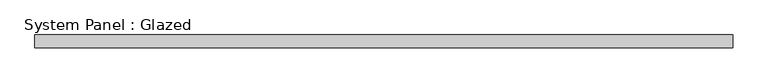
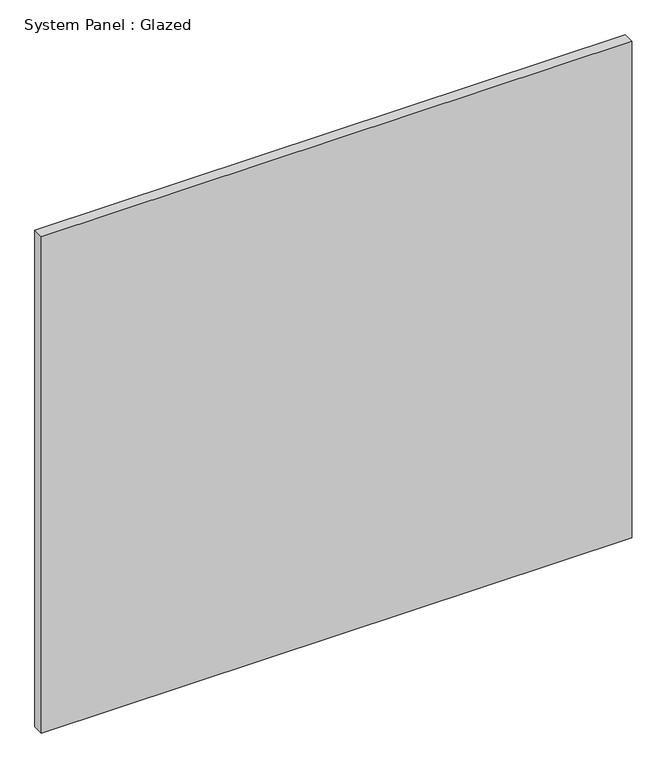
"""IFC4 building model written with IfcOpenShell, lengths in millimetres: plate geometry, System Panel : Glazed."""

from ifc_helpers import new_model, si_unit, origin, origin_with_axes, place, context, project, spatial, polyline, outline, extrude, source, transform, mapped, element, save


def system_panel_glazed_246808bb(model_context):
    return source(origin(), model_context, "Body", "SweptSolid", [
        extrude(outline(polyline([(685.8, 19.05), (-685.8, 19.05), (-685.8, 44.45), (685.8, 44.45), (685.8, 19.05)])), origin_with_axes(), (0.0, 0.0, 1.0), 1219.2),
    ])


if __name__ == "__main__":
    model = new_model("IFC4")
    model_context = context("Model", 3, world=origin())
    ifc_project = project(units=[si_unit("LENGTHUNIT", "METRE", prefix="MILLI")], contexts=[model_context])
    site = spatial("IfcSite", under=ifc_project)
    building = spatial("IfcBuilding", under=site)
    placement = place(None, origin())
    system_panel_glazed_shape = system_panel_glazed_246808bb(model_context)
    element("IfcPlate", 1, ObjectType="System Panel : Glazed", at=placement, inside=building, context=model_context, shape_type="MappedRepresentation", body=[
        mapped(system_panel_glazed_shape, transform((0.0, 0.0, 0.0), x_axis=(1.0, 0.0, 0.0), y_axis=(0.0, 1.0, 0.0), z_axis=(0.0, 0.0, 1.0))),
    ])
    save(model, "model.ifc")

# Revit data of these elements
# Type "System Panel : Glazed"
#   Construction Type Id = "GSP4R"
#   Analytic Construction = "1/8 in Pilkington single glazing"
#   Visual Light Transmittance = 0.9
#   Solar Heat Gain Coefficient = 0.86
#   Heat Transfer Coefficient (U) = 1.18115 BTU/(h·ft²·°F)
# Element 1 (IfcPlate, "System Panel : Glazed")
#   Materials on its faces: "Glass"
# Materials
#   "Glass": class "Glass", colour RGB 0 128 192, transparency 0.75, Description = "Soda Lime Glass", Cost = 0
